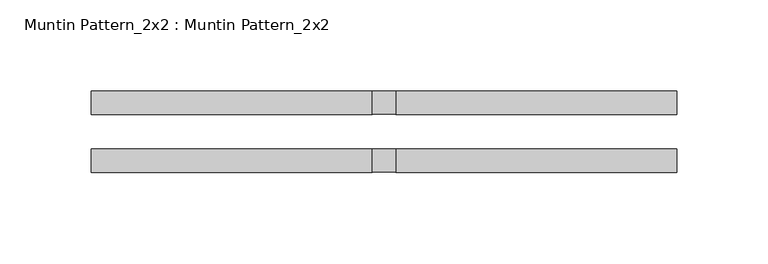
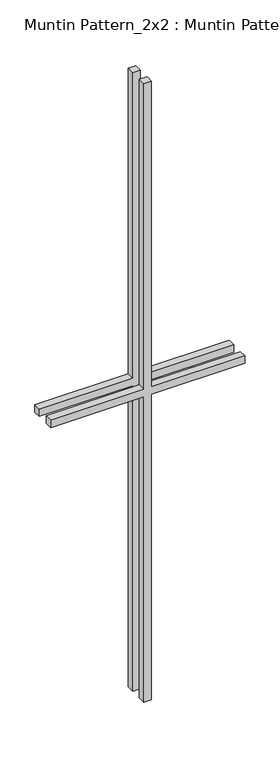
"""IFC4 building model written with IfcOpenShell, lengths in millimetres: proxy geometry, Muntin Pattern_2x2 : Muntin Pattern_2x2."""

from ifc_helpers import new_model, si_unit, frame, origin, place, context, project, spatial, polyline, outline, extrude, source, transform, mapped, element, save


def muntin_pattern_2x2_muntin_pattern_2x2_43d02eee(model_context):
    return source(origin(), model_context, "Body", "SweptSolid", [
        extrude(outline(polyline([(546.1, -6.35), (546.1, -160.3375), (533.4, -160.3375), (533.4, -6.35), (0.0, -6.35), (0.0, 6.35), (533.4, 6.35), (533.4, 160.3375), (546.1, 160.3375), (546.1, 6.35), (1079.5, 6.35), (1079.5, -6.35), (546.1, -6.35)])), frame((0.0, -22.225, 0.0), z_axis=(0.0, 1.0, 0.0), x_axis=(0.0, 0.0, 1.0)), (0.0, 0.0, 1.0), 12.7),
        extrude(outline(polyline([(546.1, -6.35), (546.1, -160.3375), (533.4, -160.3375), (533.4, -6.35), (0.0, -6.35), (0.0, 6.35), (533.4, 6.35), (533.4, 160.3375), (546.1, 160.3375), (546.1, 6.35), (1079.5, 6.35), (1079.5, -6.35), (546.1, -6.35)])), frame((0.0, 9.525, 0.0), z_axis=(0.0, 1.0, 0.0), x_axis=(0.0, 0.0, 1.0)), (0.0, 0.0, 1.0), 12.7),
    ])


if __name__ == "__main__":
    model = new_model("IFC4")
    model_context = context("Model", 3, world=origin())
    ifc_project = project(units=[si_unit("LENGTHUNIT", "METRE", prefix="MILLI")], contexts=[model_context])
    site = spatial("IfcSite", under=ifc_project)
    building = spatial("IfcBuilding", under=site)
    placement = place(None, origin())
    muntin_pattern_2x2_muntin_pattern_2x2_shape = muntin_pattern_2x2_muntin_pattern_2x2_43d02eee(model_context)
    element("IfcBuildingElementProxy", 1, Name="Muntin Pattern_2x2 : Muntin Pattern_2x2", ObjectType="Muntin Pattern_2x2 : Muntin Pattern_2x2", at=placement, inside=building, context=model_context, shape_type="MappedRepresentation", body=[
        mapped(muntin_pattern_2x2_muntin_pattern_2x2_shape, transform((0.0, 0.0, 0.0), x_axis=(1.0, 0.0, 0.0), y_axis=(0.0, 1.0, 0.0), z_axis=(0.0, 0.0, 1.0))),
    ])
    save(model, "model.ifc")

# Revit data of these elements
# Type "Muntin Pattern_2x2 : Muntin Pattern_2x2"
#   Width [instance default] = 4' - 0"
#   Thickness = 0' - 0 1/2"
#   Height [instance default] = 4' - 0"
#   Distance = 0' - 0 3/4"
#   Interior Material [instance default] = none
#   Exterior Material [instance default] = none
#   Default Elevation = 0
# Element 1 (IfcBuildingElementProxy, "Muntin Pattern_2x2 : Muntin Pattern_2x2")
#   Width = 1' - 0 5/8"
#   Height = 3' - 6 1/2"
#   Interior Material = Wood - Stained
#   Exterior Material = Clad - White
#   Materials on its faces: "Clad - White", "Wood - Stained"
# Materials
#   "Clad - White": class "Wood", colour RGB 242 242 238, transparency 0, Cost = 0
#   "Wood - Stained": class "Wood", colour RGB 224 178 126, transparency 0, Cost = 0
